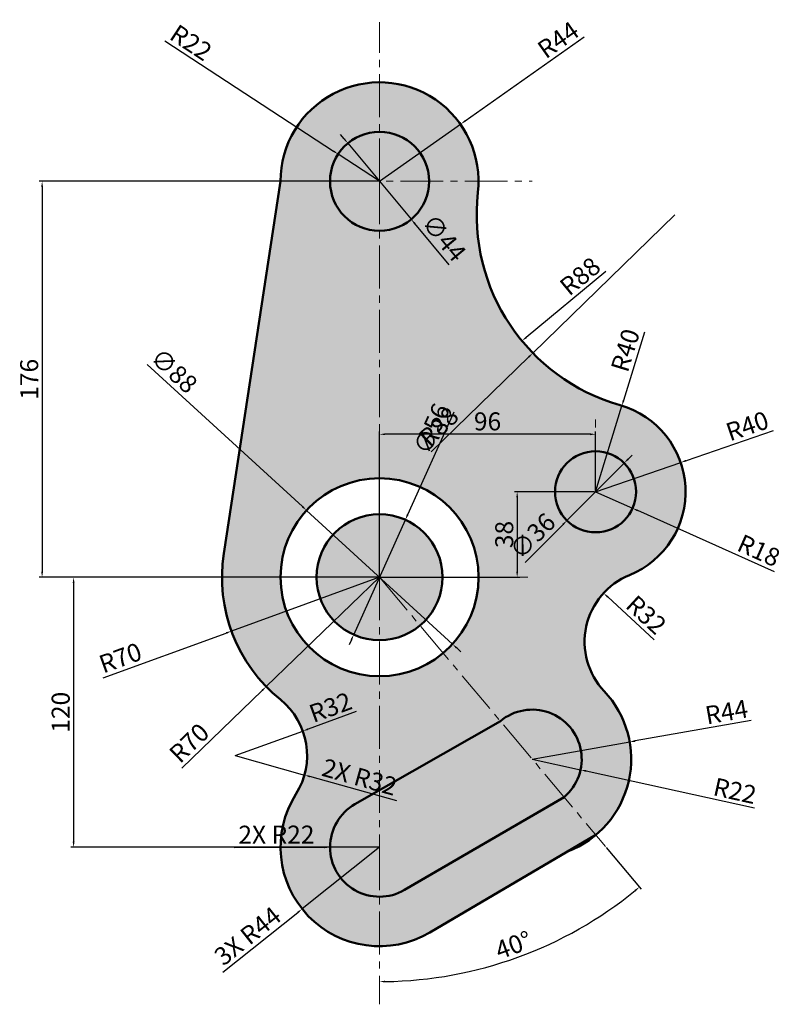
# Model space of a CAD drawing. Units: millimetres. Extents: x 3107 to 3446, y 1917 to 2355.
import ezdxf

# ---------------------------------------------------------------- set-up
doc = ezdxf.new("R2010")
doc.units = ezdxf.units.MM
doc.linetypes.add('CENTER2', pattern=[28.575, 19.05, -3.175, 3.175, -3.175])
for name, color, linetype, lineweight in [('M-CNTR', 10, 'CENTER2', 18), ('M-DIMS', 2, 'Continuous', 25), ('M-HATC', 8, 'Continuous', 18), ('M-OUTL', 7, 'Continuous', 50)]:
    doc.layers.add(name, color=color, linetype=linetype, lineweight=lineweight)
doc.styles.get("Standard").update_dxf_attribs({"font": 'arial.ttf'})
doc.dimstyles.new('ISO-25', dxfattribs={"dimtxt": 8, "dimasz": 2.5, "dimexe": 1.25, "dimexo": 0.625, "dimtad": 1, "dimtxsty": 'Standard', "dimcen": 2.5, "dimadec": 0, "dimazin": 0, "dimtfac": 1, "dimtmove": 0, "dimatfit": 3, "dimfxl": 1, "dimarcsym": 0})

# ---------------------------------------------------------------- blocks, each defined once
blk = doc.blocks.new('*D1')
at = {"layer": 'Defpoints', "color": 0, "transparency": 16777216}
for p in [(3266.8, 2107.24), (3266.8, 1987.24), (3367.17, 1987.62), (3308.25, 1932.37), (3266.8, 1917.42)]:
    blk.add_point(p, dxfattribs=at)
at = {"layer": 'M-DIMS', "color": 0, "lineweight": -2, "transparency": 16777216}
blk.add_line((3367.57, 1987.15), (3383.12, 1968.61), dxfattribs=at)
blk.add_arc((3266.8, 2107.24), 179.72, 270.797, 309.203, dxfattribs=at)
at = {"layer": 'M-DIMS', "color": 0, "transparency": 16777216}
for points in [[(3380.13, 1968.3), (3380.66, 1967.65), (3382.32, 1969.57)], [(3269.3, 1927.12), (3269.3, 1927.96), (3266.8, 1927.52)]]:
    blk.add_solid(points, dxfattribs=at)
at = {"layer": 'M-DIMS', "color": 0, "transparency": 16777216, "insert": (3326.66, 1942.79), "char_height": 8, "attachment_point": 5, "rotation": 20}
blk.add_mtext('40°', dxfattribs=at)
blk = doc.blocks.new('*D2')
at = {"layer": 'Defpoints', "color": 0, "transparency": 16777216}
for p in [(3334.63, 2026.41), (3356.11, 2021.66)]:
    blk.add_point(p, dxfattribs=at)
at = {"layer": 'M-DIMS', "color": 0, "lineweight": -2, "transparency": 16777216}
for p, q in [((3334.63, 2026.41), (3356.11, 2021.66)), ((3433.4, 2004.58), (3358.55, 2021.12))]:
    blk.add_line(p, q, dxfattribs=at)
at = {"layer": 'M-DIMS', "color": 0, "transparency": 16777216}
blk.add_solid([(3358.64, 2021.53), (3358.46, 2020.71), (3356.11, 2021.66)], dxfattribs=at)
at = {"layer": 'M-DIMS', "color": 0, "transparency": 16777216, "insert": (3424.5, 2011.3), "char_height": 8, "attachment_point": 5, "rotation": 347.5405}
blk.add_mtext('R22', dxfattribs=at)
blk = doc.blocks.new('*D3')
at = {"layer": 'Defpoints', "color": 0, "transparency": 16777216}
for p in [(3377.96, 2034.04), (3334.63, 2026.41)]:
    blk.add_point(p, dxfattribs=at)
at = {"layer": 'M-DIMS', "color": 0, "lineweight": -2, "transparency": 16777216}
for p, q in [((3432.01, 2043.57), (3380.42, 2034.48)), ((3334.63, 2026.41), (3377.96, 2034.04))]:
    blk.add_line(p, q, dxfattribs=at)
at = {"layer": 'M-DIMS', "color": 0, "transparency": 16777216}
blk.add_solid([(3380.35, 2034.89), (3380.5, 2034.07), (3377.96, 2034.04)], dxfattribs=at)
at = {"layer": 'M-DIMS', "color": 0, "transparency": 16777216, "insert": (3421.19, 2046.36), "char_height": 8, "attachment_point": 5, "rotation": 9.996}
blk.add_mtext('R44', dxfattribs=at)
blk = doc.blocks.new('*D4')
at = {"layer": 'Defpoints', "color": 0, "transparency": 16777216}
for p in [(3366.35, 2100.19), (3389.92, 2078.55)]:
    blk.add_point(p, dxfattribs=at)
at = {"layer": 'M-DIMS', "color": 0, "lineweight": -2, "transparency": 16777216}
blk.add_line((3388.89, 2079.49), (3368.19, 2098.5), dxfattribs=at)
at = {"layer": 'M-DIMS', "color": 0, "transparency": 16777216}
blk.add_solid([(3368.47, 2098.8), (3367.91, 2098.19), (3366.35, 2100.19)], dxfattribs=at)
at = {"layer": 'M-DIMS', "color": 0, "transparency": 16777216, "insert": (3384.61, 2089.82), "char_height": 8, "attachment_point": 5, "rotation": 317.4528}
blk.add_mtext('R32', dxfattribs=at)
blk = doc.blocks.new('*D5')
at = {"layer": 'Defpoints', "color": 0, "transparency": 16777216}
for p in [(3362.8, 2145.24), (3379.23, 2137.9)]:
    blk.add_point(p, dxfattribs=at)
at = {"layer": 'M-DIMS', "color": 0, "lineweight": -2, "transparency": 16777216}
for p, q in [((3362.8, 2145.24), (3379.23, 2137.9)), ((3442.32, 2109.72), (3381.52, 2136.88))]:
    blk.add_line(p, q, dxfattribs=at)
at = {"layer": 'M-DIMS', "color": 0, "transparency": 16777216}
blk.add_solid([(3381.69, 2137.26), (3381.35, 2136.5), (3379.23, 2137.9)], dxfattribs=at)
at = {"layer": 'M-DIMS', "color": 0, "transparency": 16777216, "insert": (3434.94, 2118.18), "char_height": 8, "attachment_point": 5, "rotation": 335.9299}
blk.add_mtext('R18', dxfattribs=at)
blk = doc.blocks.new('*D6')
at = {"layer": 'Defpoints', "color": 0, "transparency": 16777216}
for p in [(3302.76, 2308.6), (3266.8, 2283.24)]:
    blk.add_point(p, dxfattribs=at)
at = {"layer": 'M-DIMS', "color": 0, "lineweight": -2, "transparency": 16777216}
for p, q in [((3357.76, 2347.38), (3304.8, 2310.04)), ((3266.8, 2283.24), (3302.76, 2308.6))]:
    blk.add_line(p, q, dxfattribs=at)
at = {"layer": 'M-DIMS', "color": 0, "transparency": 16777216}
blk.add_solid([(3304.56, 2310.38), (3305.04, 2309.7), (3302.76, 2308.6)], dxfattribs=at)
at = {"layer": 'M-DIMS', "color": 0, "transparency": 16777216, "insert": (3346.78, 2345.3), "char_height": 8, "attachment_point": 5, "rotation": 35.1866}
blk.add_mtext('R44', dxfattribs=at)
blk = doc.blocks.new('*D7')
at = {"layer": 'Defpoints', "color": 0, "transparency": 16777216}
for p in [(3248.4, 2295.3), (3266.8, 2283.24)]:
    blk.add_point(p, dxfattribs=at)
at = {"layer": 'M-DIMS', "color": 0, "lineweight": -2, "transparency": 16777216}
for p, q in [((3171.44, 2345.71), (3246.3, 2296.67)), ((3266.8, 2283.24), (3248.4, 2295.3))]:
    blk.add_line(p, q, dxfattribs=at)
at = {"layer": 'M-DIMS', "color": 0, "transparency": 16777216}
blk.add_solid([(3246.53, 2297.02), (3246.08, 2296.32), (3248.4, 2295.3)], dxfattribs=at)
at = {"layer": 'M-DIMS', "color": 0, "transparency": 16777216, "insert": (3182.47, 2344.04), "char_height": 8, "attachment_point": 5, "rotation": 326.7714}
blk.add_mtext('R22', dxfattribs=at)
blk = doc.blocks.new('*D8')
at = {"layer": 'Defpoints', "color": 0, "transparency": 16777216}
for p in [(3397.95, 2268.32), (3330.1, 2212.28)]:
    blk.add_point(p, dxfattribs=at)
at = {"layer": 'M-DIMS', "color": 0, "lineweight": -2, "transparency": 16777216}
blk.add_line((3367.43, 2243.11), (3332.03, 2213.88), dxfattribs=at)
at = {"layer": 'M-DIMS', "color": 0, "transparency": 16777216}
blk.add_solid([(3331.76, 2214.2), (3332.29, 2213.55), (3330.1, 2212.28)], dxfattribs=at)
at = {"layer": 'M-DIMS', "color": 0, "transparency": 16777216, "insert": (3356.57, 2240.25), "char_height": 8, "attachment_point": 5, "rotation": 39.5529}
blk.add_mtext('R88', dxfattribs=at)
blk = doc.blocks.new('*D9')
at = {"layer": 'Defpoints', "color": 0, "transparency": 16777216}
for p in [(3232.71, 2038.88), (3202.63, 2027.96)]:
    blk.add_point(p, dxfattribs=at)
at = {"layer": 'M-DIMS', "color": 0, "lineweight": -2, "transparency": 16777216}
for p, q in [((3256.47, 2047.51), (3235.06, 2039.73)), ((3202.63, 2027.96), (3232.71, 2038.88))]:
    blk.add_line(p, q, dxfattribs=at)
at = {"layer": 'M-DIMS', "color": 0, "transparency": 16777216}
blk.add_solid([(3234.91, 2040.12), (3235.2, 2039.34), (3232.71, 2038.88)], dxfattribs=at)
at = {"layer": 'M-DIMS', "color": 0, "transparency": 16777216, "insert": (3245.33, 2048.48), "char_height": 8, "attachment_point": 5, "rotation": 19.9513}
blk.add_mtext('R32', dxfattribs=at)
blk = doc.blocks.new('*D10')
at = {"layer": 'Defpoints', "color": 0, "transparency": 16777216}
for p in [(3266.8, 2107.24), (3201.02, 2083.3)]:
    blk.add_point(p, dxfattribs=at)
at = {"layer": 'M-DIMS', "color": 0, "lineweight": -2, "transparency": 16777216}
for p, q in [((3266.8, 2107.24), (3201.02, 2083.3)), ((3144.03, 2062.55), (3198.67, 2082.44))]:
    blk.add_line(p, q, dxfattribs=at)
at = {"layer": 'M-DIMS', "color": 0, "transparency": 16777216}
blk.add_solid([(3198.53, 2082.83), (3198.82, 2082.05), (3201.02, 2083.3)], dxfattribs=at)
at = {"layer": 'M-DIMS', "color": 0, "transparency": 16777216, "insert": (3151.98, 2070.45), "char_height": 8, "attachment_point": 5, "rotation": 20.0049}
blk.add_mtext('R70', dxfattribs=at)
blk = doc.blocks.new('*D11')
at = {"layer": 'Defpoints', "color": 0, "transparency": 16777216}
for p in [(3234.36, 2136.97), (3299.23, 2077.51)]:
    blk.add_point(p, dxfattribs=at)
at = {"layer": 'M-DIMS', "color": 0, "lineweight": -2, "transparency": 16777216}
for p, q in [((3163.57, 2201.86), (3232.52, 2138.66)), ((3299.23, 2077.51), (3234.36, 2136.97)), ((3301.08, 2075.82), (3302.92, 2074.13))]:
    blk.add_line(p, q, dxfattribs=at)
at = {"layer": 'M-DIMS', "color": 0, "transparency": 16777216}
for points in [[(3232.8, 2138.97), (3232.24, 2138.36), (3234.36, 2136.97)], [(3301.36, 2076.13), (3300.8, 2075.52), (3299.23, 2077.51)]]:
    blk.add_solid(points, dxfattribs=at)
at = {"layer": 'M-DIMS', "color": 0, "transparency": 16777216, "insert": (3174.8, 2198.26), "char_height": 8, "attachment_point": 5, "rotation": 317.4924}
blk.add_mtext('∅88', dxfattribs=at)
blk = doc.blocks.new('*D12')
at = {"layer": 'Defpoints', "color": 0, "transparency": 16777216}
for p in [(3278.28, 2132.78), (3255.32, 2081.71)]:
    blk.add_point(p, dxfattribs=at)
at = {"layer": 'M-DIMS', "color": 0, "lineweight": -2, "transparency": 16777216}
for p, q in [((3299.76, 2180.56), (3279.3, 2135.06)), ((3255.32, 2081.71), (3278.28, 2132.78)), ((3254.29, 2079.43), (3253.27, 2077.15))]:
    blk.add_line(p, q, dxfattribs=at)
at = {"layer": 'M-DIMS', "color": 0, "transparency": 16777216}
for points in [[(3278.92, 2135.23), (3279.68, 2134.89), (3278.28, 2132.78)], [(3253.91, 2079.6), (3254.67, 2079.25), (3255.32, 2081.71)]]:
    blk.add_solid(points, dxfattribs=at)
at = {"layer": 'M-DIMS', "color": 0, "transparency": 16777216, "insert": (3290.87, 2172.82), "char_height": 8, "attachment_point": 5, "rotation": 65.7924}
blk.add_mtext('∅56', dxfattribs=at)
blk = doc.blocks.new('*D13')
at = {"layer": 'Defpoints', "color": 0, "transparency": 16777216}
for p in [(3400.63, 2158.24), (3362.8, 2145.24)]:
    blk.add_point(p, dxfattribs=at)
at = {"layer": 'M-DIMS', "color": 0, "lineweight": -2, "transparency": 16777216}
for p, q in [((3441.69, 2172.35), (3402.99, 2159.06)), ((3362.8, 2145.24), (3400.63, 2158.24))]:
    blk.add_line(p, q, dxfattribs=at)
at = {"layer": 'M-DIMS', "color": 0, "transparency": 16777216}
blk.add_solid([(3402.86, 2159.45), (3403.13, 2158.66), (3400.63, 2158.24)], dxfattribs=at)
at = {"layer": 'M-DIMS', "color": 0, "transparency": 16777216, "insert": (3430.54, 2173.5), "char_height": 8, "attachment_point": 5, "rotation": 18.9663}
blk.add_mtext('R40', dxfattribs=at)
blk = doc.blocks.new('*D14')
at = {"layer": 'Defpoints', "color": 0, "transparency": 16777216}
for p in [(3266.8, 2170.79), (3362.8, 2145.24), (3266.8, 2107.24)]:
    blk.add_point(p, dxfattribs=at)
at = {"layer": 'M-DIMS', "color": 0, "lineweight": -2, "transparency": 16777216}
for p, q in [((3266.8, 2107.87), (3266.8, 2172.04)), ((3360.3, 2170.79), (3269.3, 2170.79)), ((3362.8, 2145.87), (3362.8, 2172.04))]:
    blk.add_line(p, q, dxfattribs=at)
at = {"layer": 'M-DIMS', "color": 0, "transparency": 16777216}
for points in [[(3269.3, 2171.21), (3269.3, 2170.38), (3266.8, 2170.79)], [(3360.3, 2171.21), (3360.3, 2170.38), (3362.8, 2170.79)]]:
    blk.add_solid(points, dxfattribs=at)
at = {"layer": 'M-DIMS', "color": 0, "transparency": 16777216, "insert": (3314.8, 2175.5), "char_height": 8, "attachment_point": 5}
blk.add_mtext('96', dxfattribs=at)
blk = doc.blocks.new('*D15')
at = {"layer": 'Defpoints', "color": 0, "transparency": 16777216}
for p in [(3362.8, 2145.24), (3266.8, 2107.24), (3327.96, 2107.24)]:
    blk.add_point(p, dxfattribs=at)
at = {"layer": 'M-DIMS', "color": 0, "lineweight": -2, "transparency": 16777216}
for p, q in [((3362.17, 2145.24), (3326.71, 2145.24)), ((3327.96, 2142.74), (3327.96, 2109.74)), ((3267.42, 2107.24), (3329.21, 2107.24))]:
    blk.add_line(p, q, dxfattribs=at)
at = {"layer": 'M-DIMS', "color": 0, "transparency": 16777216}
for points in [[(3327.55, 2142.74), (3328.38, 2142.74), (3327.96, 2145.24)], [(3327.55, 2109.74), (3328.38, 2109.74), (3327.96, 2107.24)]]:
    blk.add_solid(points, dxfattribs=at)
at = {"layer": 'M-DIMS', "color": 0, "transparency": 16777216, "insert": (3323.25, 2126.24), "char_height": 8, "attachment_point": 5, "rotation": 90}
blk.add_mtext('38', dxfattribs=at)
blk = doc.blocks.new('*D16')
at = {"layer": 'Defpoints', "color": 0, "transparency": 16777216}
for p in [(3266.8, 2283.24), (3116.86, 2107.24), (3266.8, 2107.24)]:
    blk.add_point(p, dxfattribs=at)
at = {"layer": 'M-DIMS', "color": 0, "lineweight": -2, "transparency": 16777216}
for p, q in [((3266.17, 2283.24), (3115.61, 2283.24)), ((3116.86, 2280.74), (3116.86, 2109.74)), ((3266.17, 2107.24), (3115.61, 2107.24))]:
    blk.add_line(p, q, dxfattribs=at)
at = {"layer": 'M-DIMS', "color": 0, "transparency": 16777216}
for points in [[(3116.45, 2280.74), (3117.28, 2280.74), (3116.86, 2283.24)], [(3116.45, 2109.74), (3117.28, 2109.74), (3116.86, 2107.24)]]:
    blk.add_solid(points, dxfattribs=at)
at = {"layer": 'M-DIMS', "color": 0, "transparency": 16777216, "insert": (3112.15, 2195.24), "char_height": 8, "attachment_point": 5, "rotation": 90}
blk.add_mtext('176', dxfattribs=at)
blk = doc.blocks.new('*D17')
at = {"layer": 'Defpoints', "color": 0, "transparency": 16777216}
for p in [(3266.8, 2107.24), (3130.86, 1987.24), (3266.8, 1987.24)]:
    blk.add_point(p, dxfattribs=at)
at = {"layer": 'M-DIMS', "color": 0, "lineweight": -2, "transparency": 16777216}
for p, q in [((3266.17, 2107.24), (3129.61, 2107.24)), ((3130.86, 2104.74), (3130.86, 1989.74)), ((3266.17, 1987.24), (3129.61, 1987.24))]:
    blk.add_line(p, q, dxfattribs=at)
at = {"layer": 'M-DIMS', "color": 0, "transparency": 16777216}
for points in [[(3130.44, 2104.74), (3131.28, 2104.74), (3130.86, 2107.24)], [(3130.44, 1989.74), (3131.28, 1989.74), (3130.86, 1987.24)]]:
    blk.add_solid(points, dxfattribs=at)
at = {"layer": 'M-DIMS', "color": 0, "transparency": 16777216, "insert": (3126.15, 2047.24), "char_height": 8, "attachment_point": 5, "rotation": 90}
blk.add_mtext('120', dxfattribs=at)
blk = doc.blocks.new('*D18')
at = {"layer": 'Defpoints', "color": 0, "transparency": 16777216}
for p in [(3397.95, 2268.32), (3334.92, 2206.92)]:
    blk.add_point(p, dxfattribs=at)
at = {"layer": 'M-DIMS', "color": 0, "lineweight": -2, "transparency": 16777216}
for p, q in [((3397.95, 2268.32), (3334.92, 2206.92)), ((3289.79, 2162.96), (3333.12, 2205.17))]:
    blk.add_line(p, q, dxfattribs=at)
at = {"layer": 'M-DIMS', "color": 0, "transparency": 16777216}
blk.add_solid([(3332.83, 2205.47), (3333.42, 2204.88), (3334.92, 2206.92)], dxfattribs=at)
at = {"layer": 'M-DIMS', "color": 0, "transparency": 16777216, "insert": (3293.81, 2173.45), "char_height": 8, "attachment_point": 5, "rotation": 44.2481}
blk.add_mtext('R88', dxfattribs=at)
blk = doc.blocks.new('*D19')
at = {"layer": 'Defpoints', "color": 0, "transparency": 16777216}
for p in [(3266.8, 2107.24), (3216.43, 2058.63)]:
    blk.add_point(p, dxfattribs=at)
at = {"layer": 'M-DIMS', "color": 0, "lineweight": -2, "transparency": 16777216}
for p, q in [((3266.8, 2107.24), (3216.43, 2058.63)), ((3178.89, 2022.4), (3214.63, 2056.89))]:
    blk.add_line(p, q, dxfattribs=at)
at = {"layer": 'M-DIMS', "color": 0, "transparency": 16777216}
blk.add_solid([(3214.34, 2057.19), (3214.92, 2056.59), (3216.43, 2058.63)], dxfattribs=at)
at = {"layer": 'M-DIMS', "color": 0, "transparency": 16777216, "insert": (3182.94, 2032.85), "char_height": 8, "attachment_point": 5, "rotation": 43.9848}
blk.add_mtext('R70', dxfattribs=at)
blk = doc.blocks.new('*D20')
at = {"layer": 'Defpoints', "color": 0, "transparency": 16777216}
for p in [(3266.8, 1987.24), (3232.4, 1959.8)]:
    blk.add_point(p, dxfattribs=at)
at = {"layer": 'M-DIMS', "color": 0, "lineweight": -2, "transparency": 16777216}
for p, q in [((3266.8, 1987.24), (3232.4, 1959.8)), ((3197.1, 1931.64), (3230.45, 1958.24))]:
    blk.add_line(p, q, dxfattribs=at)
at = {"layer": 'M-DIMS', "color": 0, "transparency": 16777216}
blk.add_solid([(3230.19, 1958.57), (3230.71, 1957.92), (3232.4, 1959.8)], dxfattribs=at)
at = {"layer": 'M-DIMS', "color": 0, "transparency": 16777216, "insert": (3208.83, 1947.02), "char_height": 8, "attachment_point": 5, "rotation": 38.582}
blk.add_mtext('3X R44', dxfattribs=at)
blk = doc.blocks.new('*D21')
at = {"layer": 'Defpoints', "color": 0, "transparency": 16777216}
for p in [(3374.5, 2183.49), (3362.8, 2145.24)]:
    blk.add_point(p, dxfattribs=at)
at = {"layer": 'M-DIMS', "color": 0, "lineweight": -2, "transparency": 16777216}
for p, q in [((3384.49, 2216.17), (3375.23, 2185.88)), ((3362.8, 2145.24), (3374.5, 2183.49))]:
    blk.add_line(p, q, dxfattribs=at)
at = {"layer": 'M-DIMS', "color": 0, "transparency": 16777216}
blk.add_solid([(3374.83, 2186.01), (3375.63, 2185.76), (3374.5, 2183.49)], dxfattribs=at)
at = {"layer": 'M-DIMS', "color": 0, "transparency": 16777216, "insert": (3377.01, 2207.82), "char_height": 8, "attachment_point": 5, "rotation": 72.9928}
blk.add_mtext('R40', dxfattribs=at)
blk = doc.blocks.new('*D22')
at = {"layer": 'Defpoints', "color": 0, "transparency": 16777216}
for p in [(3202.63, 2027.96), (3233.44, 2019.34)]:
    blk.add_point(p, dxfattribs=at)
at = {"layer": 'M-DIMS', "color": 0, "lineweight": -2, "transparency": 16777216}
for p, q in [((3202.63, 2027.96), (3233.44, 2019.34)), ((3274.48, 2007.85), (3235.85, 2018.66))]:
    blk.add_line(p, q, dxfattribs=at)
at = {"layer": 'M-DIMS', "color": 0, "transparency": 16777216}
blk.add_solid([(3235.96, 2019.06), (3235.74, 2018.26), (3233.44, 2019.34)], dxfattribs=at)
at = {"layer": 'M-DIMS', "color": 0, "transparency": 16777216, "insert": (3257.64, 2017.46), "char_height": 8, "attachment_point": 5, "rotation": 344.3663}
blk.add_mtext('2X R32', dxfattribs=at)
blk = doc.blocks.new('*D23')
at = {"layer": 'Defpoints', "color": 0, "transparency": 16777216}
for p in [(3252.72, 2300.14), (3280.88, 2266.34)]:
    blk.add_point(p, dxfattribs=at)
at = {"layer": 'M-DIMS', "color": 0, "lineweight": -2, "transparency": 16777216}
for p, q in [((3251.11, 2302.07), (3249.51, 2303.99)), ((3252.72, 2300.14), (3280.88, 2266.34)), ((3297.77, 2246.07), (3282.48, 2264.42))]:
    blk.add_line(p, q, dxfattribs=at)
at = {"layer": 'M-DIMS', "color": 0, "transparency": 16777216}
for points in [[(3251.43, 2302.33), (3250.79, 2301.8), (3252.72, 2300.14)], [(3282.8, 2264.69), (3282.16, 2264.15), (3280.88, 2266.34)]]:
    blk.add_solid(points, dxfattribs=at)
at = {"layer": 'M-DIMS', "color": 0, "transparency": 16777216, "insert": (3294.72, 2257.45), "char_height": 8, "attachment_point": 5, "rotation": 309.803}
blk.add_mtext('∅44', dxfattribs=at)
blk = doc.blocks.new('*D24')
at = {"layer": 'Defpoints', "color": 0, "transparency": 16777216}
for p in [(3244.8, 1987.2), (3266.8, 1987.24)]:
    blk.add_point(p, dxfattribs=at)
at = {"layer": 'M-DIMS', "color": 0, "lineweight": -2, "transparency": 16777216}
for p, q in [((3202.19, 1987.12), (3242.3, 1987.2)), ((3266.8, 1987.24), (3244.8, 1987.2))]:
    blk.add_line(p, q, dxfattribs=at)
at = {"layer": 'M-DIMS', "color": 0, "transparency": 16777216}
blk.add_solid([(3242.3, 1987.61), (3242.3, 1986.78), (3244.8, 1987.2)], dxfattribs=at)
at = {"layer": 'M-DIMS', "color": 0, "transparency": 16777216, "insert": (3220.98, 1991.8), "char_height": 8, "attachment_point": 5, "rotation": 0.1129}
blk.add_mtext('2X R22', dxfattribs=at)
blk = doc.blocks.new('*D25')
at = {"layer": 'Defpoints', "color": 0, "transparency": 16777216}
for p in [(3375.5, 2157.99), (3350.09, 2132.49)]:
    blk.add_point(p, dxfattribs=at)
at = {"layer": 'M-DIMS', "color": 0, "lineweight": -2, "transparency": 16777216}
for p, q in [((3375.5, 2157.99), (3350.09, 2132.49)), ((3377.27, 2159.76), (3379.03, 2161.54)), ((3331.45, 2113.79), (3348.33, 2130.72))]:
    blk.add_line(p, q, dxfattribs=at)
at = {"layer": 'M-DIMS', "color": 0, "transparency": 16777216}
for points in [[(3376.97, 2160.06), (3377.56, 2159.47), (3375.5, 2157.99)], [(3348.03, 2131.02), (3348.62, 2130.43), (3350.09, 2132.49)]]:
    blk.add_solid(points, dxfattribs=at)
at = {"layer": 'M-DIMS', "color": 0, "transparency": 16777216, "insert": (3335.51, 2124.85), "char_height": 8, "attachment_point": 5, "rotation": 45.1011}
blk.add_mtext('∅36', dxfattribs=at)

msp = doc.modelspace()

# ---------------------------------------------------------------- hatches: boundary and pattern name
at = {"layer": 'M-HATC'}
h = msp.add_hatch(color=256, dxfattribs=at)
h.set_gradient(color1=(0, 255, 0), color2=(255, 255, 0), tint=1)
h.paths.add_polyline_path([(3197.597, 2117.784, 0.2664219), (3222.758, 2052.833, -0.3809002), (3229.646, 2010.816, 0.7872114), (3289.095, 1949.311), (3362.912, 1992.7, 0.4312911), (3366.641, 2056.593, -0.5271868), (3377.867, 2108.19, 0.7128287), (3373.784, 2183.705, -0.3666921), (3310.516, 2278.269, 1.0583107), (3222.798, 2283.243)])
h.paths.add_polyline_path([(3244.798, 2283.243, -1), (3288.798, 2283.243, -1)], flags=16)
h.paths.add_polyline_path([(3310.798, 2107.243, -1), (3222.798, 2107.243, -1)], flags=16)
h.paths.add_polyline_path([(3294.798, 2107.243, -1), (3238.798, 2107.243, -1)], flags=0)
h.paths.add_polyline_path([(3380.798, 2145.243, -1), (3344.798, 2145.243, -1)], flags=16)
h.paths.add_polyline_path([(3348.771, 2009.553), (3277.876, 1968.236, -1.0042892), (3255.884, 2006.345), (3320.488, 2043.259, -1)], flags=16)
h = msp.add_hatch(color=256, dxfattribs=at)
h.set_gradient(color1=(205, 105, 40), color2=(255, 255, 0), tint=1, name='SPHERICAL')
h.paths.add_polyline_path([(3244.798, 2283.243, 1), (3288.798, 2283.243, 1)])
h = msp.add_hatch(color=256, dxfattribs=at)
h.set_gradient(color1=(205, 105, 40), color2=(255, 255, 0), tint=1, name='SPHERICAL')
h.paths.add_polyline_path([(3344.798, 2145.243, 1), (3380.798, 2145.243, 1)])
h = msp.add_hatch(color=256, dxfattribs=at)
h.set_gradient(color1=(205, 105, 40), color2=(255, 255, 0), tint=1, name='SPHERICAL')
h.paths.add_polyline_path([(3238.798, 2107.243, 1), (3294.798, 2107.243, 1)])
h = msp.add_hatch(color=256, dxfattribs=at)
h.set_gradient(color1=(205, 105, 40), color2=(255, 255, 0), tint=1, name='SPHERICAL')
h.paths.add_polyline_path([(3348.771, 2009.553, 1), (3320.488, 2043.259), (3255.884, 2006.345, 1.0042892), (3277.876, 1968.236)])

# ---------------------------------------------------------------- linework, layer by layer
at = {"layer": 'M-CNTR'}
for p, q in [((3266.798, 2283.243), (3266.798, 2354.031)), ((3190.358, 2283.243), (3334.611, 2283.243)), ((3266.798, 2283.243), (3266.798, 2107.243)), ((3362.798, 2145.243), (3362.798, 2177.334)), ((3362.798, 2145.243), (3331.043, 2145.243)), ((3143.295, 2107.243), (3332.63, 2107.243)), ((3266.798, 2107.243), (3266.798, 1987.243)), ((3266.798, 2107.243), (3367.17, 1987.625)), ((3266.798, 1987.243), (3266.798, 1917.423))]:
    msp.add_line(p, q, dxfattribs=at)
at = {"layer": 'M-OUTL'}
for p, q in [((3222.798, 2283.243), (3197.597, 2117.784)), ((3320.488, 2043.259), (3255.884, 2006.345)), ((3348.771, 2009.553), (3277.876, 1968.236)), ((3362.912, 1992.7), (3289.095, 1949.311))]:
    msp.add_line(p, q, dxfattribs=at)
for centre, radius in [((3266.798, 2283.243), 22), ((3362.798, 2145.243), 18), ((3266.798, 2107.243), 44), ((3266.798, 2107.243), 28)]:
    msp.add_circle(centre, radius, dxfattribs=at)
for centre, radius, start, end in [((3266.798, 2283.243), 44, 353.50912, 180), ((3397.952, 2268.321), 88, 173.50912, 254.05947), ((3362.798, 2145.243), 40, 292.13001, 74.05947), ((3266.798, 2107.243), 70, 171.33959, 231.0129), ((3389.922, 2078.548), 32, 112.13001, 223.32044), ((3202.626, 2027.96), 32, 327.60551, 51.0129), ((3334.629, 2026.406), 44, 290.89282, 43.32044), ((3334.629, 2026.406), 22, 310, 130), ((3266.798, 1987.243), 44, 147.60551, 300.44641), ((3266.798, 1987.243), 22, 119.7428, 300.23325)]:
    msp.add_arc(centre, radius, start, end, dxfattribs=at)

# ---------------------------------------------------------------- dimensions: what is measured, and where the dimension line sits
at = {"layer": 'M-DIMS'}
for center, mpoint, override, picture, middle in [((3266.798, 2283.243), (3302.759, 2308.598), {"dimclrd": 0, "dimclre": 0, "dimclrt": 0}, '*D6', (3349.448, 2341.517)), ((3266.798, 2283.243), (3248.396, 2295.299), {"dimclrd": 0, "dimclre": 0, "dimclrt": 0}, '*D7', (3179.922, 2340.156)), ((3397.952, 2268.321), (3334.916, 2206.918), {"dimdec": 0, "dimlfac": 1, "dimrnd": 0, "dimzin": 0, "dimdsep": 46, "dimlunit": 2}, '*D18', (3297.094, 2170.076)), ((3397.952, 2268.321), (3330.101, 2212.284), {"dimclrd": 0, "dimclre": 0, "dimclrt": 0}, '*D8', (3359.569, 2236.621)), ((3362.798, 2145.243), (3374.498, 2183.494), {"dimdec": 0, "dimlfac": 1, "dimrnd": 0, "dimzin": 0, "dimdsep": 46, "dimlunit": 2}, '*D21', (3381.518, 2206.445)), ((3362.798, 2145.243), (3400.627, 2158.244), {"dimclrd": 0, "dimclre": 0, "dimclrt": 0}, '*D13', (3432.068, 2169.049)), ((3362.798, 2145.243), (3379.233, 2137.902), {"dimclrd": 0, "dimclre": 0, "dimclrt": 0}, '*D5', (3433.018, 2113.877)), ((3266.798, 2107.243), (3201.022, 2083.296), {"dimclrd": 0, "dimclre": 0, "dimclrt": 0}, '*D10', (3153.591, 2066.028)), ((3266.798, 2107.243), (3216.432, 2058.631), {"dimdec": 0, "dimlfac": 1, "dimrnd": 0, "dimzin": 0, "dimdsep": 46, "dimlunit": 2}, '*D19', (3186.212, 2029.463)), ((3389.922, 2078.548), (3366.347, 2100.186), {"dimclrd": 0, "dimclre": 0, "dimclrt": 0}, '*D4', (3381.422, 2086.349)), ((3334.629, 2026.406), (3377.962, 2034.043), {"dimclrd": 0, "dimclre": 0, "dimclrt": 0}, '*D3', (3421.997, 2041.805)), ((3334.629, 2026.406), (3356.111, 2021.659), {"dimclrd": 0, "dimclre": 0, "dimclrt": 0}, '*D2', (3423.5, 2006.769))]:
    dim = msp.add_radius_dim(center=center, mpoint=mpoint, dimstyle='ISO-25', override=override, dxfattribs=at)
    dim.commit()
    dim.dimension.update_dxf_attribs({"geometry": picture, "text_midpoint": middle, "dimtype": 164})
for p1, p2, override, picture, middle in [((3252.715, 2300.145), (3280.882, 2266.342), {"dimdec": 0, "dimlfac": 1, "dimrnd": 0, "dimzin": 0, "dimdsep": 46, "dimlunit": 2}, '*D23', (3290.926, 2254.288)), ((3299.235, 2077.513), (3234.362, 2136.974), {"dimclrd": 0, "dimclre": 0, "dimclrt": 0}, '*D11', (3171.467, 2194.622)), ((3255.317, 2081.706), (3278.28, 2132.781), {"dimclrd": 0, "dimclre": 0, "dimclrt": 0}, '*D12', (3295.369, 2170.793))]:
    dim = msp.add_diameter_dim_2p(p1=p1, p2=p2, dimstyle='ISO-25', override=override, dxfattribs=at)
    dim.commit()
    dim.dimension.update_dxf_attribs({"geometry": picture, "text_midpoint": middle, "dimtype": 163})
for base, p1, p2, picture, middle in [((3116.863, 2107.243), (3266.798, 2283.243), (3266.798, 2107.243), '*D16', (3112.153, 2195.243)), ((3327.962, 2107.243), (3362.798, 2145.243), (3266.798, 2107.243), '*D15', (3323.25, 2126.243)), ((3130.862, 1987.243), (3266.798, 2107.243), (3266.798, 1987.243), '*D17', (3126.152, 2047.243))]:
    dim = msp.add_linear_dim(base=base, p1=p1, p2=p2, angle=90, dimstyle='ISO-25', override={"dimclrd": 0, "dimclre": 0, "dimclrt": 0}, dxfattribs=at)
    dim.commit()
    dim.dimension.update_dxf_attribs({"geometry": picture, "text_midpoint": middle})
dim = msp.add_linear_dim(base=(3266.798, 2170.793), p1=(3362.798, 2145.243), p2=(3266.798, 2107.243), dimstyle='ISO-25', override={"dimclrd": 0, "dimclre": 0, "dimclrt": 0}, dxfattribs=at)
dim.commit()
dim.dimension.update_dxf_attribs({"geometry": '*D14', "text_midpoint": (3314.798, 2175.502)})
dim = msp.add_diameter_dim_2p(p1=(3375.504, 2157.994), p2=(3350.093, 2132.493), dimstyle='ISO-25', override={"dimdec": 0, "dimlfac": 1, "dimrnd": 0, "dimzin": 0, "dimdsep": 46, "dimlunit": 2}, dxfattribs=at)
dim.commit()
dim.dimension.update_dxf_attribs({"geometry": '*D25', "text_midpoint": (3339.008, 2121.369)})
dim = msp.add_angular_dim_2l(base=(3308.245, 1932.366), line1=((3266.798, 2107.243), (3367.17, 1987.625)), line2=((3266.798, 1987.243), (3266.798, 1917.423)), dimstyle='ISO-25', override={"dimclrd": 0, "dimclre": 0, "dimclrt": 0}, dxfattribs=at)
dim.commit()
dim.dimension.update_dxf_attribs({"geometry": '*D1', "text_midpoint": (3326.656, 1942.786)})
dim = msp.add_radius_dim(center=(3202.626, 2027.96), mpoint=(3232.705, 2038.879), dimstyle='ISO-25', override={"dimclrd": 0, "dimclre": 0, "dimclrt": 0}, dxfattribs=at)
dim.commit()
dim.dimension.update_dxf_attribs({"geometry": '*D9', "text_midpoint": (3245.33, 2048.475)})
for center, mpoint, picture, middle in [((3202.626, 2027.96), (3233.442, 2019.336), '*D22', (3257.636, 2017.459)), ((3266.798, 1987.243), (3244.799, 1987.2), '*D24', (3220.984, 1991.797))]:
    dim = msp.add_radius_dim(center=center, mpoint=mpoint, text='2X <>', dimstyle='ISO-25', override={"dimdec": 0, "dimlfac": 1, "dimrnd": 0, "dimzin": 0, "dimdsep": 46, "dimlunit": 2}, dxfattribs=at)
    dim.commit()
    dim.dimension.update_dxf_attribs({"geometry": picture, "text_midpoint": middle})
dim = msp.add_radius_dim(center=(3266.798, 1987.243), mpoint=(3232.403, 1959.803), text='3X <>', dimstyle='ISO-25', override={"dimdec": 0, "dimlfac": 1, "dimrnd": 0, "dimzin": 0, "dimdsep": 46, "dimlunit": 2}, dxfattribs=at)
dim.commit()
dim.dimension.update_dxf_attribs({"geometry": '*D20', "text_midpoint": (3211.766, 1943.34), "dimtype": 164})

doc.saveas('drawing.dxf')
